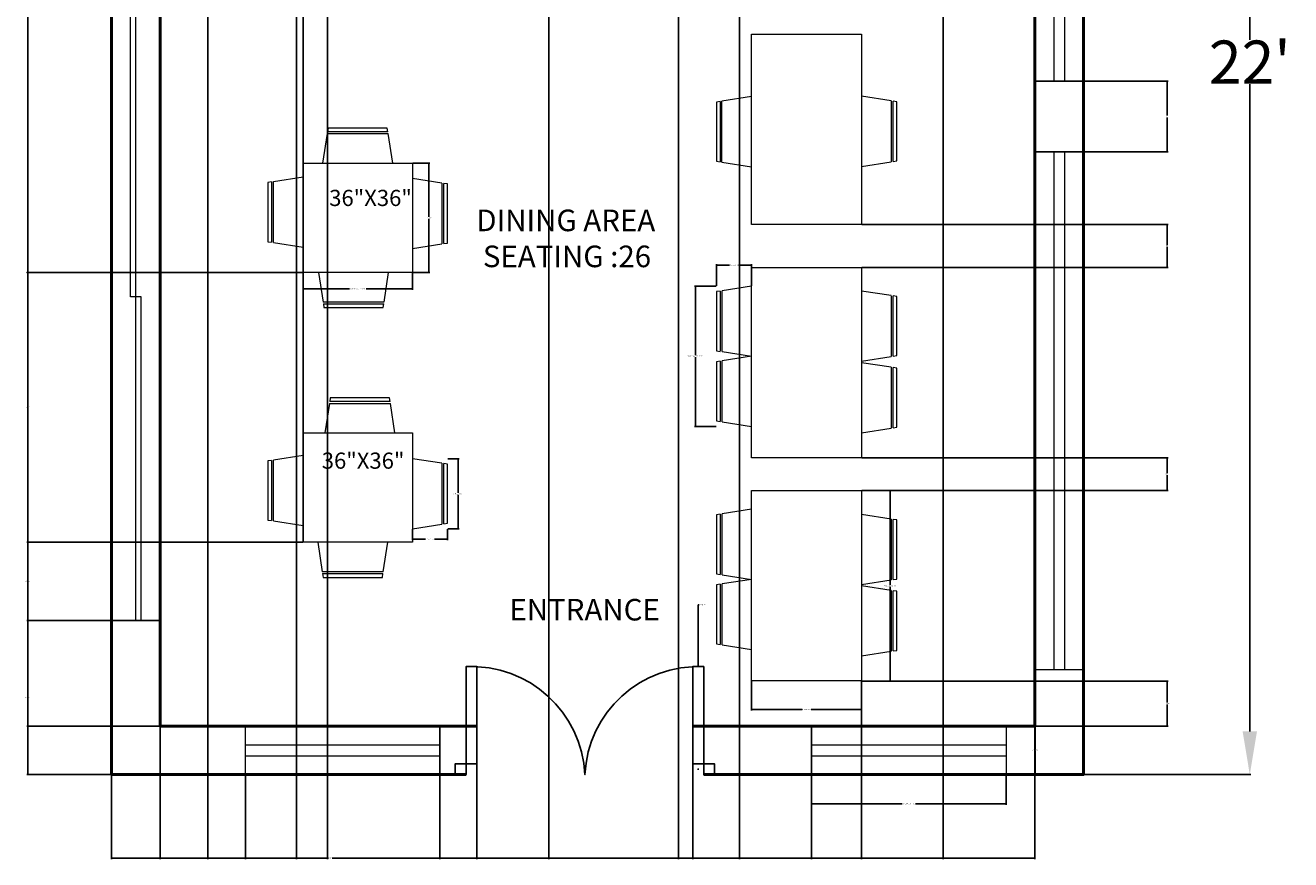
# Model space of a CAD drawing. Units: inches. Extents: x 226 to 1155, y 22 to 494.
# Tile 1 of 7: x 226 to 460, y 22 to 176. Entities that reach past the tile are written whole.
import ezdxf

# ---------------------------------------------------------------- set-up
doc = ezdxf.new("R2010")
doc.units = ezdxf.units.IN
doc.header["$MEASUREMENT"] = 0
for name, color, linetype, lineweight in [('A-ANNO-DIMS', 2, 'Continuous', 18), ('A-ANNO-TEXT', 7, 'Continuous', 18), ('A-AREA-IDEN', 7, 'Continuous', 25), ('A-DOOR', 3, 'Continuous', 25), ('A-FURN', 8, 'Continuous', 18), ('A-GLAZ', 4, 'Continuous', 18), ('A-WALL', 7, 'Continuous', 50)]:
    doc.layers.add(name, color=color, linetype=linetype, lineweight=lineweight)
doc.styles.get("Standard").update_dxf_attribs({"font": 'arial.ttf'})
doc.dimstyles.get("Standard").update_dxf_attribs({"dimtxt": 0.18, "dimasz": 0.18, "dimexe": 0.18, "dimexo": 0.0625, "dimgap": 0.09, "dimtad": 0, "dimtih": 1, "dimtoh": 1, "dimdec": 4, "dimzin": 0, "dimdsep": 46, "dimlunit": 4, "dimtxsty": 'Standard', "dimcen": 0.09, "dimadec": 0, "dimazin": 0, "dimtfac": 1, "dimtdec": 4, "dimtofl": 0, "dimtmove": 0, "dimatfit": 3, "dimfxl": 1, "dimtolj": 1, "dimtzin": 0, "dimarcsym": 0})

# ---------------------------------------------------------------- blocks, each defined once
blk = doc.blocks.new('*D8')
at = {"layer": 'A-ANNO-DIMS', "color": 0, "lineweight": -2, "transparency": 16777216}
for p, q in [((421.77, 301.63), (452.71, 301.63)), ((452.53, 293.63), (452.53, 173.74)), ((452.53, 45.63), (452.53, 165.52)), ((421.77, 37.63), (452.71, 37.63))]:
    blk.add_line(p, q, dxfattribs=at)
at = {"layer": 'A-ANNO-DIMS', "color": 0, "transparency": 16777216}
for points in [[(451.2, 293.63), (453.86, 293.63), (452.53, 301.63)], [(451.2, 45.63), (453.86, 45.63), (452.53, 37.63)]]:
    blk.add_solid(points, dxfattribs=at)
at = {"layer": 'Defpoints', "color": 0, "transparency": 16777216}
for p in [(421.71, 301.63), (421.71, 37.63), (452.53, 37.63)]:
    blk.add_point(p, dxfattribs=at)
at = {"layer": 'A-ANNO-DIMS', "color": 0, "transparency": 16777216, "insert": (452.53, 169.63), "char_height": 8, "attachment_point": 5}
blk.add_mtext("\\A1;22'", dxfattribs=at)
blk = doc.blocks.new('CHAIR-DINING')
for p, q in [((5.48, 12.14), (0, 12.99)), ((5.48, 12.13), (5.48, 0.85)), ((5.82, 0.91), (5.82, 12.08)), ((0, 0), (5.48, 0.86))]:
    blk.add_line(p, q)
blk.add_lwpolyline([(5.82, 0.91), (6.51, 1.02), (6.51, 11.98), (5.82, 12.08)])
blk = doc.blocks.new('CHAIR-DINING-PAIRED')
for p, q in [((6.51, 25.99), (1.03, 25.13)), ((0.68, 25.08), (0.68, 13.91)), ((1.03, 13.85), (1.03, 25.13)), ((0.68, 12.08), (0.68, 0.91)), ((1.03, 0.86), (1.03, 12.14)), ((1.03, 0.86), (6.51, 0))]:
    blk.add_line(p, q)
for points in [[(0.68, 25.08), (0, 24.97), (0, 14.01), (0.68, 13.9)], [(0.68, 12.08), (0, 11.98), (0, 1.02), (0.68, 0.91)], [(1.03, 13.85), (6.51, 12.99), (1.03, 12.14)]]:
    blk.add_lwpolyline(points)
blk = doc.blocks.new('TABLE-DINING-SQ')
blk.add_lwpolyline([(0, 20.25), (20.25, 20.25), (20.25, 0), (0, 0)], close=True)
blk = doc.blocks.new('TABLE-DINING-RECT')
blk.add_lwpolyline([(0, 35.29), (20.38, 35.29), (20.38, 0), (0, 0)], close=True)
blk = doc.blocks.new('WIN-36')
for p, q in [((0, 5.5), (36, 5.5)), ((0, 3.5), (36, 3.5))]:
    blk.add_line(p, q)
blk.add_lwpolyline([(36, 9), (36, 0), (0, 0), (0, 9)], close=True)
blk = doc.blocks.new('WIN-96')
for p, q in [((3.5, 96), (3.5, 0)), ((5.5, 96), (5.5, 0))]:
    blk.add_line(p, q)
blk.add_lwpolyline([(9, 96), (9, 0), (0, 0), (0, 96)], close=True)
blk = doc.blocks.new('WIN-120-SLIDING')
blk.add_lwpolyline([(9, 0), (0, 0), (0, 120), (9, 120)], close=True)
for points in [[(5.5, 0), (5.5, 60), (4.5, 60), (3.5, 60), (3.5, 120)], [(4.5, 0), (4.5, 60), (4.5, 120)]]:
    blk.add_lwpolyline(points)
blk = doc.blocks.new('*D22')
at = {"layer": 'A-ANNO-DIMS', "color": 0, "lineweight": -2, "transparency": 16777216}
for p, q in [((304, 96.16), (306.07, 96.16)), ((305.89, 95.98), (305.89, 89.85)), ((305.89, 83.35), (305.89, 89.48)), ((304, 83.17), (306.07, 83.17))]:
    blk.add_line(p, q, dxfattribs=at)
at = {"layer": 'A-ANNO-DIMS', "color": 0, "transparency": 16777216}
for points in [[(305.86, 95.98), (305.92, 95.98), (305.89, 96.16)], [(305.86, 83.35), (305.92, 83.35), (305.89, 83.17)]]:
    blk.add_solid(points, dxfattribs=at)
at = {"layer": 'Defpoints', "color": 0, "transparency": 16777216}
for p in [(303.94, 96.16), (305.89, 96.16), (303.94, 83.17)]:
    blk.add_point(p, dxfattribs=at)
at = {"layer": 'A-ANNO-DIMS', "color": 0, "transparency": 16777216, "insert": (305.89, 89.67), "char_height": 0.18, "attachment_point": 5}
blk.add_mtext('\\A1;CHAIR 1\'-1" TYP.', dxfattribs=at)
blk = doc.blocks.new('*D23')
at = {"layer": 'A-ANNO-DIMS', "color": 0, "lineweight": -2, "transparency": 16777216}
for p, q in [((297.43, 83.11), (297.43, 81.04)), ((303.94, 83.11), (303.94, 81.04)), ((297.61, 81.22), (299.84, 81.22)), ((303.76, 81.22), (301.53, 81.22))]:
    blk.add_line(p, q, dxfattribs=at)
at = {"layer": 'A-ANNO-DIMS', "color": 0, "transparency": 16777216}
for points in [[(297.61, 81.25), (297.61, 81.19), (297.43, 81.22)], [(303.76, 81.25), (303.76, 81.19), (303.94, 81.22)]]:
    blk.add_solid(points, dxfattribs=at)
at = {"layer": 'Defpoints', "color": 0, "transparency": 16777216}
for p in [(297.43, 83.17), (303.94, 83.17), (303.94, 81.22)]:
    blk.add_point(p, dxfattribs=at)
at = {"layer": 'A-ANNO-DIMS', "color": 0, "transparency": 16777216, "insert": (300.68, 81.22), "char_height": 0.18, "attachment_point": 5}
blk.add_mtext('\\A1;0\'-6 1/2" TYP.', dxfattribs=at)
blk = doc.blocks.new('*D28')
at = {"layer": 'A-ANNO-DIMS', "color": 0, "lineweight": -2, "transparency": 16777216}
for p, q in [((380.69, 90.26), (386.1, 90.26)), ((385.92, 90.08), (385.92, 72.8)), ((385.92, 55.15), (385.92, 72.44)), ((380.69, 54.97), (386.1, 54.97))]:
    blk.add_line(p, q, dxfattribs=at)
at = {"layer": 'A-ANNO-DIMS', "color": 0, "transparency": 16777216}
for points in [[(385.89, 90.08), (385.95, 90.08), (385.92, 90.26)], [(385.89, 55.15), (385.95, 55.15), (385.92, 54.97)]]:
    blk.add_solid(points, dxfattribs=at)
at = {"layer": 'Defpoints', "color": 0, "transparency": 16777216}
for p in [(380.63, 90.26), (385.92, 90.26), (380.63, 54.97)]:
    blk.add_point(p, dxfattribs=at)
at = {"layer": 'A-ANNO-DIMS', "color": 0, "transparency": 16777216, "insert": (385.92, 72.62), "char_height": 0.18, "attachment_point": 5}
blk.add_mtext('\\A1;TABLE 2\'-11 1/2" TYP.', dxfattribs=at)
blk = doc.blocks.new('*D29')
at = {"layer": 'A-ANNO-DIMS', "color": 0, "lineweight": -2, "transparency": 16777216}
for p, q in [((360.25, 54.91), (360.25, 49.5)), ((380.63, 54.91), (380.63, 49.5)), ((360.43, 49.68), (369.6, 49.68)), ((380.45, 49.68), (371.28, 49.68))]:
    blk.add_line(p, q, dxfattribs=at)
at = {"layer": 'A-ANNO-DIMS', "color": 0, "transparency": 16777216}
for points in [[(360.43, 49.71), (360.43, 49.65), (360.25, 49.68)], [(380.45, 49.71), (380.45, 49.65), (380.63, 49.68)]]:
    blk.add_solid(points, dxfattribs=at)
at = {"layer": 'Defpoints', "color": 0, "transparency": 16777216}
for p in [(360.25, 54.97), (380.63, 54.97), (380.63, 49.68)]:
    blk.add_point(p, dxfattribs=at)
at = {"layer": 'A-ANNO-DIMS', "color": 0, "transparency": 16777216, "insert": (370.44, 49.68), "char_height": 0.18, "attachment_point": 5}
blk.add_mtext('\\A1;1\'-8 1/2" TYP.', dxfattribs=at)
blk = doc.blocks.new('*D32')
at = {"layer": 'A-ANNO-DIMS', "color": 0, "lineweight": -2, "transparency": 16777216}
for p, q in [((371.38, 37.57), (371.38, 32.05)), ((407.38, 37.57), (407.38, 32.05)), ((371.56, 32.23), (388.16, 32.23)), ((407.2, 32.23), (390.61, 32.23))]:
    blk.add_line(p, q, dxfattribs=at)
at = {"layer": 'A-ANNO-DIMS', "color": 0, "transparency": 16777216}
for points in [[(371.56, 32.26), (371.56, 32.2), (371.38, 32.23)], [(407.2, 32.26), (407.2, 32.2), (407.38, 32.23)]]:
    blk.add_solid(points, dxfattribs=at)
at = {"layer": 'Defpoints', "color": 0, "transparency": 16777216}
for p in [(371.38, 37.63), (407.38, 37.63), (407.38, 32.23)]:
    blk.add_point(p, dxfattribs=at)
at = {"layer": 'A-ANNO-DIMS', "color": 0, "transparency": 16777216, "insert": (389.38, 32.23), "char_height": 0.18, "attachment_point": 5}
blk.add_mtext('\\A1;WINDOW 3\'-0" TYP.', dxfattribs=at)
blk = doc.blocks.new('*D33')
at = {"layer": 'A-ANNO-DIMS', "color": 0, "lineweight": -2, "transparency": 16777216}
for p, q in [((407.45, 46.63), (412.96, 46.63)), ((412.78, 46.45), (412.78, 42.31)), ((412.78, 37.81), (412.78, 41.95)), ((407.45, 37.63), (412.96, 37.63))]:
    blk.add_line(p, q, dxfattribs=at)
at = {"layer": 'A-ANNO-DIMS', "color": 0, "transparency": 16777216}
for points in [[(412.75, 46.45), (412.81, 46.45), (412.78, 46.63)], [(412.75, 37.81), (412.81, 37.81), (412.78, 37.63)]]:
    blk.add_solid(points, dxfattribs=at)
at = {"layer": 'Defpoints', "color": 0, "transparency": 16777216}
for p in [(407.38, 46.63), (412.78, 46.63), (407.38, 37.63)]:
    blk.add_point(p, dxfattribs=at)
at = {"layer": 'A-ANNO-DIMS', "color": 0, "transparency": 16777216, "insert": (412.78, 42.13), "char_height": 0.18, "attachment_point": 5}
blk.add_mtext('\\A1;0\'-9" TYP.', dxfattribs=at)
blk = doc.blocks.new('*D34')
at = {"layer": 'A-ANNO-DIMS', "color": 0, "lineweight": -2, "transparency": 16777216}
for p, q in [((353.68, 128.13), (349.67, 128.13)), ((349.85, 127.95), (349.85, 115.32)), ((349.85, 102.32), (349.85, 114.95)), ((353.68, 102.14), (349.67, 102.14))]:
    blk.add_line(p, q, dxfattribs=at)
at = {"layer": 'A-ANNO-DIMS', "color": 0, "transparency": 16777216}
for points in [[(349.82, 127.95), (349.88, 127.95), (349.85, 128.13)], [(349.82, 102.32), (349.88, 102.32), (349.85, 102.14)]]:
    blk.add_solid(points, dxfattribs=at)
at = {"layer": 'Defpoints', "color": 0, "transparency": 16777216}
for p in [(349.85, 128.13), (353.74, 128.13), (353.74, 102.14)]:
    blk.add_point(p, dxfattribs=at)
at = {"layer": 'A-ANNO-DIMS', "color": 0, "transparency": 16777216, "insert": (349.85, 115.14), "char_height": 0.18, "attachment_point": 5}
blk.add_mtext('\\A1;PAIRED CHAIRS 2\'-2" TYP.', dxfattribs=at)
blk = doc.blocks.new('*D35')
at = {"layer": 'A-ANNO-DIMS', "color": 0, "lineweight": -2, "transparency": 16777216}
for p, q in [((353.74, 128.19), (353.74, 132.21)), ((353.92, 132.03), (356.15, 132.03)), ((360.07, 132.03), (357.85, 132.03)), ((360.25, 128.19), (360.25, 132.21))]:
    blk.add_line(p, q, dxfattribs=at)
at = {"layer": 'A-ANNO-DIMS', "color": 0, "transparency": 16777216}
for points in [[(353.92, 132.06), (353.92, 132), (353.74, 132.03)], [(360.07, 132.06), (360.07, 132), (360.25, 132.03)]]:
    blk.add_solid(points, dxfattribs=at)
at = {"layer": 'Defpoints', "color": 0, "transparency": 16777216}
for p in [(360.25, 132.03), (353.74, 128.13), (360.25, 128.13)]:
    blk.add_point(p, dxfattribs=at)
at = {"layer": 'A-ANNO-DIMS', "color": 0, "transparency": 16777216, "insert": (357, 132.03), "char_height": 0.18, "attachment_point": 5}
blk.add_mtext('\\A1;0\'-6 1/2" TYP.', dxfattribs=at)
blk = doc.blocks.new('*D40')
at = {"layer": 'A-ANNO-DIMS', "color": 0, "lineweight": -2, "transparency": 16777216}
for p, q in [((277.18, 130.6), (277.18, 127.45)), ((297.43, 130.6), (297.43, 127.45)), ((277.36, 127.63), (285.77, 127.63)), ((297.25, 127.63), (288.84, 127.63))]:
    blk.add_line(p, q, dxfattribs=at)
at = {"layer": 'A-ANNO-DIMS', "color": 0, "transparency": 16777216}
for points in [[(277.36, 127.66), (277.36, 127.6), (277.18, 127.63)], [(297.25, 127.66), (297.25, 127.6), (297.43, 127.63)]]:
    blk.add_solid(points, dxfattribs=at)
at = {"layer": 'Defpoints', "color": 0, "transparency": 16777216}
for p in [(277.18, 130.67), (297.43, 130.67), (297.43, 127.63)]:
    blk.add_point(p, dxfattribs=at)
at = {"layer": 'A-ANNO-DIMS', "color": 0, "transparency": 16777216, "insert": (287.31, 127.63), "char_height": 0.18, "attachment_point": 5}
blk.add_mtext('\\A1;TABLE BLOCK 1\'-8" TYP.', dxfattribs=at)
blk = doc.blocks.new('*D41')
at = {"layer": 'A-ANNO-DIMS', "color": 0, "lineweight": -2, "transparency": 16777216}
for p, q in [((297.49, 150.91), (300.65, 150.91)), ((300.47, 150.73), (300.47, 140.97)), ((300.47, 130.85), (300.47, 140.61)), ((297.49, 130.67), (300.65, 130.67))]:
    blk.add_line(p, q, dxfattribs=at)
at = {"layer": 'A-ANNO-DIMS', "color": 0, "transparency": 16777216}
for points in [[(300.44, 150.73), (300.5, 150.73), (300.47, 150.91)], [(300.44, 130.85), (300.5, 130.85), (300.47, 130.67)]]:
    blk.add_solid(points, dxfattribs=at)
at = {"layer": 'Defpoints', "color": 0, "transparency": 16777216}
for p in [(297.43, 150.91), (300.47, 150.91), (297.43, 130.67)]:
    blk.add_point(p, dxfattribs=at)
at = {"layer": 'A-ANNO-DIMS', "color": 0, "transparency": 16777216, "insert": (300.47, 140.79), "char_height": 0.18, "attachment_point": 5}
blk.add_mtext('\\A1;1\'-8" TYP.', dxfattribs=at)
blk = doc.blocks.new('*D61')
at = {"layer": 'A-ANNO-DIMS', "color": 0, "lineweight": -2, "transparency": 16777216}
for p, q in [((309.38, 46.57), (309.38, 21.95)), ((349.38, 46.57), (349.38, 21.95)), ((309.56, 22.13), (329.05, 22.13)), ((349.2, 22.13), (329.71, 22.13))]:
    blk.add_line(p, q, dxfattribs=at)
at = {"layer": 'A-ANNO-DIMS', "color": 0, "transparency": 16777216}
for points in [[(309.56, 22.16), (309.56, 22.1), (309.38, 22.13)], [(349.2, 22.16), (349.2, 22.1), (349.38, 22.13)]]:
    blk.add_solid(points, dxfattribs=at)
at = {"layer": 'Defpoints', "color": 0, "transparency": 16777216}
for p in [(309.38, 46.63), (349.38, 46.63), (349.38, 22.13)]:
    blk.add_point(p, dxfattribs=at)
at = {"layer": 'A-ANNO-DIMS', "color": 0, "transparency": 16777216, "insert": (329.38, 22.13), "char_height": 0.18, "attachment_point": 5}
blk.add_mtext('\\A1;3\'-4"', dxfattribs=at)
blk = doc.blocks.new('*D62')
at = {"layer": 'A-ANNO-DIMS', "color": 0, "lineweight": -2, "transparency": 16777216}
for p, q in [((241.71, 37.57), (241.71, 21.95)), ((266.49, 37.57), (266.49, 21.95)), ((241.89, 22.13), (253.77, 22.13)), ((266.31, 22.13), (254.43, 22.13))]:
    blk.add_line(p, q, dxfattribs=at)
at = {"layer": 'A-ANNO-DIMS', "color": 0, "transparency": 16777216}
for points in [[(241.89, 22.16), (241.89, 22.1), (241.71, 22.13)], [(266.31, 22.16), (266.31, 22.1), (266.49, 22.13)]]:
    blk.add_solid(points, dxfattribs=at)
at = {"layer": 'Defpoints', "color": 0, "transparency": 16777216}
for p in [(241.71, 37.63), (266.49, 37.63), (266.49, 22.13)]:
    blk.add_point(p, dxfattribs=at)
at = {"layer": 'A-ANNO-DIMS', "color": 0, "transparency": 16777216, "insert": (254.1, 22.13), "char_height": 0.18, "attachment_point": 5}
blk.add_mtext('\\A1;2\'-1"', dxfattribs=at)
blk = doc.blocks.new('*D63')
at = {"layer": 'A-ANNO-DIMS', "color": 0, "lineweight": -2, "transparency": 16777216}
for p, q in [((302.49, 46.57), (302.49, 21.95)), ((309.38, 46.57), (309.38, 21.95)), ((302.67, 22.13), (305.6, 22.13)), ((309.2, 22.13), (306.26, 22.13))]:
    blk.add_line(p, q, dxfattribs=at)
at = {"layer": 'A-ANNO-DIMS', "color": 0, "transparency": 16777216}
for points in [[(302.67, 22.16), (302.67, 22.1), (302.49, 22.13)], [(309.2, 22.16), (309.2, 22.1), (309.38, 22.13)]]:
    blk.add_solid(points, dxfattribs=at)
at = {"layer": 'Defpoints', "color": 0, "transparency": 16777216}
for p in [(302.49, 46.63), (309.38, 46.63), (309.38, 22.13)]:
    blk.add_point(p, dxfattribs=at)
at = {"layer": 'A-ANNO-DIMS', "color": 0, "transparency": 16777216, "insert": (305.93, 22.13), "char_height": 0.18, "attachment_point": 5}
blk.add_mtext('\\A1;0\'-7"', dxfattribs=at)
blk = doc.blocks.new('*D64')
at = {"layer": 'A-ANNO-DIMS', "color": 0, "lineweight": -2, "transparency": 16777216}
for p, q in [((349.38, 46.57), (349.38, 21.95)), ((371.38, 46.57), (371.38, 21.95)), ((349.56, 22.13), (359.99, 22.13)), ((371.2, 22.13), (360.77, 22.13))]:
    blk.add_line(p, q, dxfattribs=at)
at = {"layer": 'A-ANNO-DIMS', "color": 0, "transparency": 16777216}
for points in [[(349.56, 22.16), (349.56, 22.1), (349.38, 22.13)], [(371.2, 22.16), (371.2, 22.1), (371.38, 22.13)]]:
    blk.add_solid(points, dxfattribs=at)
at = {"layer": 'Defpoints', "color": 0, "transparency": 16777216}
for p in [(349.38, 46.63), (371.38, 46.63), (371.38, 22.13)]:
    blk.add_point(p, dxfattribs=at)
at = {"layer": 'A-ANNO-DIMS', "color": 0, "transparency": 16777216, "insert": (360.38, 22.13), "char_height": 0.18, "attachment_point": 5}
blk.add_mtext('\\A1;1\'-10"', dxfattribs=at)
blk = doc.blocks.new('*D65')
at = {"layer": 'A-ANNO-DIMS', "color": 0, "lineweight": -2, "transparency": 16777216}
for p, q in [((241.64, 66.17), (226.03, 66.17)), ((226.21, 65.99), (226.21, 52.08)), ((226.21, 37.81), (226.21, 51.72)), ((241.64, 37.63), (226.03, 37.63))]:
    blk.add_line(p, q, dxfattribs=at)
at = {"layer": 'A-ANNO-DIMS', "color": 0, "transparency": 16777216}
for points in [[(226.18, 65.99), (226.24, 65.99), (226.21, 66.17)], [(226.18, 37.81), (226.24, 37.81), (226.21, 37.63)]]:
    blk.add_solid(points, dxfattribs=at)
at = {"layer": 'Defpoints', "color": 0, "transparency": 16777216}
for p in [(226.21, 66.17), (241.71, 66.17), (241.71, 37.63)]:
    blk.add_point(p, dxfattribs=at)
at = {"layer": 'A-ANNO-DIMS', "color": 0, "transparency": 16777216, "insert": (226.21, 51.9), "char_height": 0.18, "attachment_point": 5}
blk.add_mtext('\\A1;2\'-4 1/2"', dxfattribs=at)
blk = doc.blocks.new('*D67')
at = {"layer": 'A-ANNO-DIMS', "color": 0, "lineweight": -2, "transparency": 16777216}
for p, q in [((250.64, 214.63), (226.03, 214.63)), ((226.21, 214.45), (226.21, 130.81)), ((226.21, 46.81), (226.21, 130.45)), ((250.64, 46.63), (226.03, 46.63))]:
    blk.add_line(p, q, dxfattribs=at)
at = {"layer": 'A-ANNO-DIMS', "color": 0, "transparency": 16777216}
for points in [[(226.18, 214.45), (226.24, 214.45), (226.21, 214.63)], [(226.18, 46.81), (226.24, 46.81), (226.21, 46.63)]]:
    blk.add_solid(points, dxfattribs=at)
at = {"layer": 'Defpoints', "color": 0, "transparency": 16777216}
for p in [(226.21, 214.63), (250.71, 214.63), (250.71, 46.63)]:
    blk.add_point(p, dxfattribs=at)
at = {"layer": 'A-ANNO-DIMS', "color": 0, "transparency": 16777216, "insert": (226.21, 130.63), "char_height": 0.18, "attachment_point": 5}
blk.add_mtext('\\A1;14\'-0"', dxfattribs=at)
blk = doc.blocks.new('*D68')
at = {"layer": 'A-ANNO-DIMS', "color": 0, "lineweight": -2, "transparency": 16777216}
for p, q in [((277.12, 130.67), (226.03, 130.67)), ((226.21, 130.49), (226.21, 105.86)), ((226.21, 80.87), (226.21, 105.5)), ((277.12, 80.69), (226.03, 80.69))]:
    blk.add_line(p, q, dxfattribs=at)
at = {"layer": 'A-ANNO-DIMS', "color": 0, "transparency": 16777216}
for points in [[(226.18, 130.49), (226.24, 130.49), (226.21, 130.67)], [(226.18, 80.87), (226.24, 80.87), (226.21, 80.69)]]:
    blk.add_solid(points, dxfattribs=at)
at = {"layer": 'Defpoints', "color": 0, "transparency": 16777216}
for p in [(226.21, 130.67), (277.18, 130.67), (277.18, 80.69)]:
    blk.add_point(p, dxfattribs=at)
at = {"layer": 'A-ANNO-DIMS', "color": 0, "transparency": 16777216, "insert": (226.21, 105.68), "char_height": 0.18, "attachment_point": 5}
blk.add_mtext('\\A1;4\'-2"', dxfattribs=at)
blk = doc.blocks.new('*D69')
at = {"layer": 'A-ANNO-DIMS', "color": 0, "lineweight": -2, "transparency": 16777216}
for p, q in [((250.71, 46.69), (250.71, 317.31)), ((250.89, 317.13), (263.4, 317.13)), ((277, 317.13), (264.48, 317.13)), ((277.18, 80.75), (277.18, 317.31))]:
    blk.add_line(p, q, dxfattribs=at)
at = {"layer": 'A-ANNO-DIMS', "color": 0, "transparency": 16777216}
for points in [[(250.89, 317.16), (250.89, 317.1), (250.71, 317.13)], [(277, 317.16), (277, 317.1), (277.18, 317.13)]]:
    blk.add_solid(points, dxfattribs=at)
at = {"layer": 'Defpoints', "color": 0, "transparency": 16777216}
for p in [(277.18, 317.13), (277.18, 80.69), (250.71, 46.63)]:
    blk.add_point(p, dxfattribs=at)
at = {"layer": 'A-ANNO-DIMS', "color": 0, "transparency": 16777216, "insert": (263.94, 317.13), "char_height": 0.18, "attachment_point": 5}
blk.add_mtext('\\A1;2\'-2 1/2"', dxfattribs=at)
blk = doc.blocks.new('*D70')
at = {"layer": 'A-ANNO-DIMS', "color": 0, "lineweight": -2, "transparency": 16777216}
for p, q in [((380.63, 54.91), (380.63, 21.95)), ((412.71, 46.57), (412.71, 21.95)), ((380.81, 22.13), (396.34, 22.13)), ((412.53, 22.13), (397, 22.13))]:
    blk.add_line(p, q, dxfattribs=at)
at = {"layer": 'A-ANNO-DIMS', "color": 0, "transparency": 16777216}
for points in [[(380.81, 22.16), (380.81, 22.1), (380.63, 22.13)], [(412.53, 22.16), (412.53, 22.1), (412.71, 22.13)]]:
    blk.add_solid(points, dxfattribs=at)
at = {"layer": 'Defpoints', "color": 0, "transparency": 16777216}
for p in [(380.63, 54.97), (412.71, 46.63), (412.71, 22.13)]:
    blk.add_point(p, dxfattribs=at)
at = {"layer": 'A-ANNO-DIMS', "color": 0, "transparency": 16777216, "insert": (396.67, 22.13), "char_height": 0.18, "attachment_point": 5}
blk.add_mtext('\\A1;2\'-8"', dxfattribs=at)
blk = doc.blocks.new('*D71')
at = {"layer": 'A-ANNO-DIMS', "color": 0, "lineweight": -2, "transparency": 16777216}
for p, q in [((241.71, 301.57), (241.71, 21.95)), ((322.71, 301.57), (322.71, 21.95)), ((241.89, 22.13), (281.88, 22.13)), ((322.53, 22.13), (282.54, 22.13))]:
    blk.add_line(p, q, dxfattribs=at)
at = {"layer": 'A-ANNO-DIMS', "color": 0, "transparency": 16777216}
for points in [[(241.89, 22.16), (241.89, 22.1), (241.71, 22.13)], [(322.53, 22.16), (322.53, 22.1), (322.71, 22.13)]]:
    blk.add_solid(points, dxfattribs=at)
at = {"layer": 'Defpoints', "color": 0, "transparency": 16777216}
for p in [(241.71, 301.63), (322.71, 301.63), (322.71, 22.13)]:
    blk.add_point(p, dxfattribs=at)
at = {"layer": 'A-ANNO-DIMS', "color": 0, "transparency": 16777216, "insert": (282.21, 22.13), "char_height": 0.18, "attachment_point": 5}
blk.add_mtext('\\A1;6\'-9"', dxfattribs=at)
blk = doc.blocks.new('*D72')
at = {"layer": 'A-ANNO-DIMS', "color": 0, "lineweight": -2, "transparency": 16777216}
for p, q in [((322.71, 301.57), (322.71, 21.95)), ((346.71, 301.57), (346.71, 21.95)), ((322.89, 22.13), (334.38, 22.13)), ((346.53, 22.13), (335.04, 22.13))]:
    blk.add_line(p, q, dxfattribs=at)
at = {"layer": 'A-ANNO-DIMS', "color": 0, "transparency": 16777216}
for points in [[(322.89, 22.16), (322.89, 22.1), (322.71, 22.13)], [(346.53, 22.16), (346.53, 22.1), (346.71, 22.13)]]:
    blk.add_solid(points, dxfattribs=at)
at = {"layer": 'Defpoints', "color": 0, "transparency": 16777216}
for p in [(322.71, 301.63), (346.71, 301.63), (346.71, 22.13)]:
    blk.add_point(p, dxfattribs=at)
at = {"layer": 'A-ANNO-DIMS', "color": 0, "transparency": 16777216, "insert": (334.71, 22.13), "char_height": 0.18, "attachment_point": 5}
blk.add_mtext('\\A1;2\'-0"', dxfattribs=at)
blk = doc.blocks.new('*D73')
at = {"layer": 'A-ANNO-DIMS', "color": 0, "lineweight": -2, "transparency": 16777216}
for p, q in [((380.69, 54.97), (437.39, 54.97)), ((437.21, 54.79), (437.21, 50.98)), ((437.21, 46.81), (437.21, 50.62)), ((412.77, 46.63), (437.39, 46.63))]:
    blk.add_line(p, q, dxfattribs=at)
at = {"layer": 'A-ANNO-DIMS', "color": 0, "transparency": 16777216}
for points in [[(437.18, 54.79), (437.24, 54.79), (437.21, 54.97)], [(437.18, 46.81), (437.24, 46.81), (437.21, 46.63)]]:
    blk.add_solid(points, dxfattribs=at)
at = {"layer": 'Defpoints', "color": 0, "transparency": 16777216}
for p in [(380.63, 54.97), (437.21, 54.97), (412.71, 46.63)]:
    blk.add_point(p, dxfattribs=at)
at = {"layer": 'A-ANNO-DIMS', "color": 0, "transparency": 16777216, "insert": (437.21, 50.8), "char_height": 0.18, "attachment_point": 5}
blk.add_mtext('\\A1;0\'-8 1/2"', dxfattribs=at)
blk = doc.blocks.new('*D74')
at = {"layer": 'A-ANNO-DIMS', "color": 0, "lineweight": -2, "transparency": 16777216}
for p, q in [((380.69, 96.31), (437.39, 96.31)), ((437.21, 96.13), (437.21, 93.47)), ((437.21, 90.44), (437.21, 93.1)), ((380.69, 90.26), (437.39, 90.26))]:
    blk.add_line(p, q, dxfattribs=at)
at = {"layer": 'A-ANNO-DIMS', "color": 0, "transparency": 16777216}
for points in [[(437.18, 96.13), (437.24, 96.13), (437.21, 96.31)], [(437.18, 90.44), (437.24, 90.44), (437.21, 90.26)]]:
    blk.add_solid(points, dxfattribs=at)
at = {"layer": 'Defpoints', "color": 0, "transparency": 16777216}
for p in [(380.63, 96.31), (437.21, 96.31), (380.63, 90.26)]:
    blk.add_point(p, dxfattribs=at)
at = {"layer": 'A-ANNO-DIMS', "color": 0, "transparency": 16777216, "insert": (437.21, 93.28), "char_height": 0.18, "attachment_point": 5}
blk.add_mtext('\\A1;0\'-6"', dxfattribs=at)
blk = doc.blocks.new('*D75')
at = {"layer": 'A-ANNO-DIMS', "color": 0, "lineweight": -2, "transparency": 16777216}
for p, q in [((380.69, 139.55), (437.39, 139.55)), ((437.21, 139.37), (437.21, 135.75)), ((437.21, 131.78), (437.21, 135.39)), ((380.69, 131.6), (437.39, 131.6))]:
    blk.add_line(p, q, dxfattribs=at)
at = {"layer": 'A-ANNO-DIMS', "color": 0, "transparency": 16777216}
for points in [[(437.18, 139.37), (437.24, 139.37), (437.21, 139.55)], [(437.18, 131.78), (437.24, 131.78), (437.21, 131.6)]]:
    blk.add_solid(points, dxfattribs=at)
at = {"layer": 'Defpoints', "color": 0, "transparency": 16777216}
for p in [(380.63, 139.55), (437.21, 139.55), (380.63, 131.6)]:
    blk.add_point(p, dxfattribs=at)
at = {"layer": 'A-ANNO-DIMS', "color": 0, "transparency": 16777216, "insert": (437.21, 135.57), "char_height": 0.18, "attachment_point": 5}
blk.add_mtext('\\A1;0\'-8"', dxfattribs=at)
blk = doc.blocks.new('*D76')
at = {"layer": 'A-ANNO-DIMS', "color": 0, "lineweight": -2, "transparency": 16777216}
for p, q in [((412.77, 166.11), (437.39, 166.11)), ((437.21, 165.93), (437.21, 159.74)), ((437.21, 153.19), (437.21, 159.38)), ((412.77, 153.01), (437.39, 153.01))]:
    blk.add_line(p, q, dxfattribs=at)
at = {"layer": 'A-ANNO-DIMS', "color": 0, "transparency": 16777216}
for points in [[(437.18, 165.93), (437.24, 165.93), (437.21, 166.11)], [(437.18, 153.19), (437.24, 153.19), (437.21, 153.01)]]:
    blk.add_solid(points, dxfattribs=at)
at = {"layer": 'Defpoints', "color": 0, "transparency": 16777216}
for p in [(412.71, 166.11), (437.21, 166.11), (412.71, 153.01)]:
    blk.add_point(p, dxfattribs=at)
at = {"layer": 'A-ANNO-DIMS', "color": 0, "transparency": 16777216, "insert": (437.21, 159.56), "char_height": 0.18, "attachment_point": 5}
blk.add_mtext('\\A1;1\'-1"', dxfattribs=at)
blk = doc.blocks.new('*D77')
at = {"layer": 'A-ANNO-DIMS', "color": 0, "lineweight": -2, "transparency": 16777216}
for p, q in [((277.12, 80.69), (226.03, 80.69)), ((226.21, 80.51), (226.21, 73.61)), ((226.21, 66.35), (226.21, 73.24)), ((250.64, 66.17), (226.03, 66.17))]:
    blk.add_line(p, q, dxfattribs=at)
at = {"layer": 'A-ANNO-DIMS', "color": 0, "transparency": 16777216}
for points in [[(226.18, 80.51), (226.24, 80.51), (226.21, 80.69)], [(226.18, 66.35), (226.24, 66.35), (226.21, 66.17)]]:
    blk.add_solid(points, dxfattribs=at)
at = {"layer": 'Defpoints', "color": 0, "transparency": 16777216}
for p in [(226.21, 80.69), (277.18, 80.69), (250.71, 66.17)]:
    blk.add_point(p, dxfattribs=at)
at = {"layer": 'A-ANNO-DIMS', "color": 0, "transparency": 16777216, "insert": (226.21, 73.43), "char_height": 0.18, "attachment_point": 5}
blk.add_mtext('\\A1;1\'-2 1/2"', dxfattribs=at)
blk = doc.blocks.new('*D79')
at = {"layer": 'A-ANNO-DIMS', "color": 0, "lineweight": -2, "transparency": 16777216}
for p, q in [((250.71, 186.1), (250.71, 21.95)), ((259.54, 180.86), (259.54, 21.95)), ((250.89, 22.13), (254.79, 22.13)), ((259.36, 22.13), (255.45, 22.13))]:
    blk.add_line(p, q, dxfattribs=at)
at = {"layer": 'A-ANNO-DIMS', "color": 0, "transparency": 16777216}
for points in [[(250.89, 22.16), (250.89, 22.1), (250.71, 22.13)], [(259.36, 22.16), (259.36, 22.1), (259.54, 22.13)]]:
    blk.add_solid(points, dxfattribs=at)
at = {"layer": 'Defpoints', "color": 0, "transparency": 16777216}
for p in [(250.71, 186.17), (259.54, 180.93), (259.54, 22.13)]:
    blk.add_point(p, dxfattribs=at)
at = {"layer": 'A-ANNO-DIMS', "color": 0, "transparency": 16777216, "insert": (255.12, 22.13), "char_height": 0.18, "attachment_point": 5}
blk.add_mtext('\\A1;0\'-9"', dxfattribs=at)
blk = doc.blocks.new('*D80')
at = {"layer": 'A-ANNO-DIMS', "color": 0, "lineweight": -2, "transparency": 16777216}
for p, q in [((275.98, 180.86), (275.98, 21.95)), ((281.68, 180.86), (281.68, 21.95)), ((276.16, 22.13), (278.29, 22.13)), ((281.5, 22.13), (279.37, 22.13))]:
    blk.add_line(p, q, dxfattribs=at)
at = {"layer": 'A-ANNO-DIMS', "color": 0, "transparency": 16777216}
for points in [[(276.16, 22.16), (276.16, 22.1), (275.98, 22.13)], [(281.5, 22.16), (281.5, 22.1), (281.68, 22.13)]]:
    blk.add_solid(points, dxfattribs=at)
at = {"layer": 'Defpoints', "color": 0, "transparency": 16777216}
for p in [(275.98, 180.93), (281.68, 180.93), (281.68, 22.13)]:
    blk.add_point(p, dxfattribs=at)
at = {"layer": 'A-ANNO-DIMS', "color": 0, "transparency": 16777216, "insert": (278.83, 22.13), "char_height": 0.18, "attachment_point": 5}
blk.add_mtext('\\A1;0\'-5 1/2"', dxfattribs=at)
blk = doc.blocks.new('*D81')
at = {"layer": 'A-ANNO-DIMS', "color": 0, "lineweight": -2, "transparency": 16777216}
for p, q in [((358.02, 198.75), (358.02, 21.95)), ((412.71, 198.75), (412.71, 21.95)), ((358.2, 22.13), (384.82, 22.13)), ((412.53, 22.13), (385.91, 22.13))]:
    blk.add_line(p, q, dxfattribs=at)
at = {"layer": 'A-ANNO-DIMS', "color": 0, "transparency": 16777216}
for points in [[(358.2, 22.16), (358.2, 22.1), (358.02, 22.13)], [(412.53, 22.16), (412.53, 22.1), (412.71, 22.13)]]:
    blk.add_solid(points, dxfattribs=at)
at = {"layer": 'Defpoints', "color": 0, "transparency": 16777216}
for p in [(358.02, 198.82), (412.71, 198.82), (412.71, 22.13)]:
    blk.add_point(p, dxfattribs=at)
at = {"layer": 'A-ANNO-DIMS', "color": 0, "transparency": 16777216, "insert": (385.36, 22.13), "char_height": 0.18, "attachment_point": 5}
blk.add_mtext('\\A1;4\'-6 1/2"', dxfattribs=at)
blk = doc.blocks.new('*D84')
at = {"layer": 'A-ANNO-DIMS', "color": 0, "lineweight": -2, "transparency": 16777216}
for p, q in [((412.71, 292.57), (412.71, 21.95)), ((395.71, 275.57), (395.71, 21.95)), ((395.89, 22.13), (403.89, 22.13)), ((412.53, 22.13), (404.53, 22.13))]:
    blk.add_line(p, q, dxfattribs=at)
at = {"layer": 'A-ANNO-DIMS', "color": 0, "transparency": 16777216}
for points in [[(395.89, 22.16), (395.89, 22.1), (395.71, 22.13)], [(412.53, 22.16), (412.53, 22.1), (412.71, 22.13)]]:
    blk.add_solid(points, dxfattribs=at)
at = {"layer": 'Defpoints', "color": 0, "transparency": 16777216}
for p in [(412.71, 292.63), (395.71, 275.63), (412.71, 22.13)]:
    blk.add_point(p, dxfattribs=at)
at = {"layer": 'A-ANNO-DIMS', "color": 0, "transparency": 16777216, "insert": (404.21, 22.13), "char_height": 0.18, "attachment_point": 5}
blk.add_mtext('\\A1;1\'-5"', dxfattribs=at)
blk = doc.blocks.new('*D119')
at = {"layer": 'A-ANNO-DIMS', "color": 0, "lineweight": -2, "transparency": 16777216}
for p, q in [((350.56, 69.07), (350.38, 69.07)), ((350.38, 69.07), (350.38, 57.84)), ((350.29, 38.63), (350.47, 38.63)), ((350.38, 38.54), (350.38, 38.72))]:
    blk.add_line(p, q, dxfattribs=at)
at = {"layer": 'A-ANNO-DIMS', "color": 0, "transparency": 16777216}
blk.add_solid([(350.35, 57.84), (350.41, 57.84), (350.38, 57.66)], dxfattribs=at)
at = {"layer": 'Defpoints', "color": 0, "transparency": 16777216}
for p in [(350.38, 57.66), (350.38, 38.63)]:
    blk.add_point(p, dxfattribs=at)
at = {"layer": 'A-ANNO-DIMS', "color": 0, "transparency": 16777216, "insert": (351.17, 69.07), "char_height": 0.18, "attachment_point": 5}
blk.add_mtext('\\A1;4X R1\'-7"', dxfattribs=at)

msp = doc.modelspace()

# ---------------------------------------------------------------- linework, layer by layer
at = {"layer": 'A-DOOR'}
for p, q in [((305.38052, 37.62988), (307.38052, 37.62988)), ((353.38052, 37.62988), (351.38052, 37.62988))]:
    msp.add_line(p, q, dxfattribs=at)
msp.add_lwpolyline([(349.38052, 57.62988, -0.02629759), (351.38052, 57.62988), (349.38052, 57.62988), (349.38052, 39.62988), (351.38052, 39.62988), (351.38052, 57.62988, 0.414213562), (329.38052, 37.62988, 0.414213562), (307.38052, 57.62988), (307.38052, 39.62988), (309.38052, 39.62988), (309.38052, 57.62988), (307.38052, 57.62988, -0.02629759), (309.38052, 57.62988)], format="xyb", dxfattribs=at)
for points in [[(305.38052, 37.62988), (307.38052, 37.62988), (307.38052, 39.62988), (305.38052, 39.62988)], [(329.38052, 37.62988), (329.38052, 37.62988)], [(329.38052, 37.62988), (329.38052, 37.62988)], [(353.38052, 37.62988), (351.38052, 37.62988), (351.38052, 39.62988), (353.38052, 39.62988)]]:
    msp.add_lwpolyline(points, close=True, dxfattribs=at)
at = {"layer": 'A-WALL'}
for points in [[(307.38052, 37.62988), (241.70585, 37.62988), (241.70585, 301.62988), (421.70585, 301.62988), (421.70585, 37.62988), (351.38052, 37.62988)], [(309.38052, 46.62988), (250.70585, 46.62988), (250.70585, 292.62988), (312.70585, 292.62988), (312.70585, 236.41817)], [(364.70585, 214.62988), (364.70585, 292.62988), (412.70585, 292.62988), (412.70585, 46.62988), (349.38052, 46.62988)]]:
    msp.add_lwpolyline(points, dxfattribs=at)

# ---------------------------------------------------------------- block references
at = {"layer": 'A-FURN'}
for name, p in [('TABLE-DINING-RECT', (360.252, 139.546)), ('CHAIR-DINING', (380.62783, 150.31343)), ('TABLE-DINING-SQ', (277.183, 130.666)), ('CHAIR-DINING', (297.43, 135.095)), ('TABLE-DINING-RECT', (360.252, 96.3054)), ('CHAIR-DINING-PAIRED', (353.744, 102.144)), ('CHAIR-DINING', (380.62783, 114.22795)), ('CHAIR-DINING', (380.62783, 100.95729)), ('TABLE-DINING-SQ', (277.183, 80.6867)), ('CHAIR-DINING', (297.43, 83.1705)), ('TABLE-DINING-RECT', (360.252, 54.97312)), ('CHAIR-DINING-PAIRED', (353.744, 60.81107)), ('CHAIR-DINING', (380.62783, 72.8397)), ('CHAIR-DINING', (380.62783, 59.62502))]:
    msp.add_blockref(name, p, dxfattribs=at)
for p, rotation in [((360.25217, 163.25133), 180), ((293.79231, 150.91311), 90.00000000000006), ((277.1826, 148.34092), 180), ((280.0312, 130.66571), 269.9999999999996), ((294.20244, 100.93381), 90.00000000000006), ((277.1826, 96.75753), 180), ((279.88672, 80.68641), 269.9999999999997)]:
    msp.add_blockref('CHAIR-DINING', p, dxfattribs=dict(at, rotation=rotation))
at = {"layer": 'A-GLAZ', "rotation": 270}
msp.add_blockref('WIN-36', (412.70597, 202.11457), dxfattribs=at)
at = {"layer": 'A-GLAZ'}
for name, p in [('WIN-120-SLIDING', (241.706, 66.167)), ('WIN-96', (412.706, 57.01)), ('WIN-36', (266.486, 37.63)), ('WIN-36', (371.38448, 37.63))]:
    msp.add_blockref(name, p, dxfattribs=at)

# ---------------------------------------------------------------- texts
at = {"layer": 'A-ANNO-TEXT', "char_height": 3, "attachment_point": 1}
for width, insert in [(12.1239596, (282.01805, 145.9715)), (16.7887975, (280.64093, 97.29759))]:
    msp.add_mtext_dynamic_manual_height_columns('36"X36"', width=width, gutter_width=1, heights=[0], dxfattribs=dict(at, insert=insert))
at = {"layer": 'A-AREA-IDEN', "char_height": 4, "attachment_point": 1}
for s, width, insert in [('DINING AREA\\P SEATING :26', 37.218979, (309.26491, 142.30778)), ('ENTRANCE', 33.9775973, (315.40292, 70.18136))]:
    msp.add_mtext_dynamic_manual_height_columns(s, width=width, gutter_width=1, heights=[0], dxfattribs=dict(at, insert=insert))

# ---------------------------------------------------------------- dimensions: what is measured, and where the dimension line sits
at = {"layer": 'A-ANNO-DIMS'}
for base, p1, p2, picture, middle in [((277.18287, 317.12988), (250.70585, 46.62988), (277.18287, 80.68669), '*D69', (263.94436, 317.12988)), ((322.7094, 22.12988), (241.70585, 301.62988), (322.7094, 301.62988), '*D71', (282.20762, 22.12988)), ((346.7094, 22.12988), (322.7094, 301.62988), (346.7094, 301.62988), '*D72', (334.7094, 22.12988)), ((412.70584, 22.12988), (395.70585, 275.62988), (412.70584, 292.62988), '*D84', (404.20584, 22.12988)), ((412.70584, 22.12988), (358.02219, 198.81719), (412.70584, 198.81719), '*D81', (385.36402, 22.12988)), ((259.53617, 22.12988), (250.70585, 186.1667), (259.53617, 180.92618), '*D79', (255.12101, 22.12988)), ((281.67698, 22.12988), (275.98461, 180.92618), (281.67698, 180.92618), '*D80', (278.8308, 22.12988)), ((412.70584, 22.12988), (380.62756, 54.97308), (412.70584, 46.62988), '*D70', (396.6667, 22.12988)), ((309.38052, 22.12988), (302.48629, 46.62988), (309.38052, 46.62988), '*D63', (305.9334, 22.12988)), ((349.38052, 22.12988), (309.38052, 46.62988), (349.38052, 46.62988), '*D61', (329.38052, 22.12988)), ((371.38477, 22.12988), (349.38052, 46.62988), (371.38477, 46.62988), '*D64', (360.38265, 22.12988)), ((266.48629, 22.12988), (241.70585, 37.62988), (266.48629, 37.62988), '*D62', (254.09607, 22.12988))]:
    dim = msp.add_linear_dim(base=base, p1=p1, p2=p2, dimstyle='Standard', override={"dimdec": 1, "dimlfac": 1, "dimrnd": 0, "dimzin": 1, "dimdsep": 46, "dimlunit": 4, "dimfrac": 2}, dxfattribs=at)
    dim.commit()
    dim.dimension.update_dxf_attribs({"geometry": picture, "text_midpoint": middle})
for base, p1, p2, override, picture, middle in [((452.53152, 37.62988), (421.70585, 301.62988), (421.70585, 37.62988), {"dimtxt": 8, "dimasz": 8, "dimclrd": 0, "dimclre": 0, "dimclrt": 0}, '*D8', (452.53152, 169.62988)), ((226.20585, 214.62988), (250.70585, 46.62988), (250.70585, 214.62988), {"dimdec": 1, "dimlfac": 1, "dimrnd": 0, "dimzin": 1, "dimdsep": 46, "dimlunit": 4, "dimfrac": 2}, '*D67', (226.20585, 130.62988)), ((437.20585, 166.11428), (412.70584, 153.00964), (412.70584, 166.11428), {"dimdec": 1, "dimlfac": 1, "dimrnd": 0, "dimzin": 1, "dimdsep": 46, "dimlunit": 4, "dimfrac": 2}, '*D76', (437.20585, 159.56196)), ((437.20585, 139.54596), (380.62756, 131.59608), (380.62756, 139.54596), {"dimdec": 1, "dimlfac": 1, "dimrnd": 0, "dimzin": 1, "dimdsep": 46, "dimlunit": 4, "dimfrac": 2}, '*D75', (437.20585, 135.57102)), ((226.20585, 130.66598), (277.18287, 80.68669), (277.18287, 130.66598), {"dimdec": 1, "dimlfac": 1, "dimrnd": 0, "dimzin": 1, "dimdsep": 46, "dimlunit": 4, "dimfrac": 2}, '*D68', (226.20585, 105.67634)), ((437.20585, 96.30536), (380.62756, 90.2638), (380.62756, 96.30536), {"dimdec": 1, "dimlfac": 1, "dimrnd": 0, "dimzin": 1, "dimdsep": 46, "dimlunit": 4, "dimfrac": 2}, '*D74', (437.20585, 93.28458)), ((226.20585, 80.68669), (250.70585, 66.1667), (277.18287, 80.68669), {"dimdec": 1, "dimlfac": 1, "dimrnd": 0, "dimzin": 1, "dimdsep": 46, "dimlunit": 4, "dimfrac": 2}, '*D77', (226.20585, 73.4267)), ((226.20585, 66.1667), (241.70585, 37.62988), (241.70585, 66.1667), {"dimdec": 1, "dimlfac": 1, "dimrnd": 0, "dimzin": 1, "dimdsep": 46, "dimlunit": 4, "dimfrac": 2}, '*D65', (226.20585, 51.89829)), ((437.20585, 54.97308), (412.70584, 46.62988), (380.62756, 54.97308), {"dimdec": 1, "dimlfac": 1, "dimrnd": 0, "dimzin": 1, "dimdsep": 46, "dimlunit": 4, "dimfrac": 2}, '*D73', (437.20585, 50.80148))]:
    dim = msp.add_linear_dim(base=base, p1=p1, p2=p2, angle=90, dimstyle='Standard', override=override, dxfattribs=at)
    dim.commit()
    dim.dimension.update_dxf_attribs({"geometry": picture, "text_midpoint": middle})
for base, p1, p2, text, picture, middle in [((300.46675, 150.91283), (297.42972, 130.66598), (297.42972, 150.91283), '<> TYP.', '*D41', (300.46675, 140.78941)), ((349.84586, 128.13057), (353.7438, 102.14427), (353.7438, 128.13057), 'PAIRED CHAIRS <> TYP.', '*D34', (349.84586, 115.13742)), ((305.88734, 96.16393), (303.93837, 83.17078), (303.93837, 96.16393), 'CHAIR <> TYP.', '*D22', (305.88734, 89.66735)), ((385.92116, 90.2638), (380.62756, 54.97308), (380.62756, 90.2638), 'TABLE <> TYP.', '*D28', (385.92116, 72.61844)), ((412.78477, 46.62988), (407.38477, 37.62988), (407.38477, 46.62988), '<> TYP.', '*D33', (412.78477, 42.12988))]:
    dim = msp.add_linear_dim(base=base, p1=p1, p2=p2, angle=90, text=text, dimstyle='Standard', override={"dimdec": 1, "dimlfac": 1, "dimrnd": 0, "dimzin": 1, "dimdsep": 46, "dimlunit": 4, "dimfrac": 2}, dxfattribs=at)
    dim.commit()
    dim.dimension.update_dxf_attribs({"geometry": picture, "text_midpoint": middle})
for base, p1, p2, text, picture, middle in [((360.25245, 132.02851), (353.7438, 128.13057), (360.25245, 128.13057), '<> TYP.', '*D35', (356.99813, 132.02851)), ((297.42972, 127.62896), (277.18287, 130.66598), (297.42972, 130.66598), 'TABLE BLOCK <> TYP.', '*D40', (287.3063, 127.62896)), ((303.93837, 81.22181), (297.42972, 83.17078), (303.93837, 83.17078), '<> TYP.', '*D23', (300.68405, 81.22181)), ((380.62756, 49.67948), (360.25245, 54.97308), (380.62756, 54.97308), '<> TYP.', '*D29', (370.44, 49.67948)), ((407.38477, 32.22988), (371.38477, 37.62988), (407.38477, 37.62988), 'WINDOW <> TYP.', '*D32', (389.38477, 32.22988))]:
    dim = msp.add_linear_dim(base=base, p1=p1, p2=p2, text=text, dimstyle='Standard', override={"dimdec": 1, "dimlfac": 1, "dimrnd": 0, "dimzin": 1, "dimdsep": 46, "dimlunit": 4, "dimfrac": 2}, dxfattribs=at)
    dim.commit()
    dim.dimension.update_dxf_attribs({"geometry": picture, "text_midpoint": middle})
dim = msp.add_radius_dim(center=(350.38052, 38.62988), mpoint=(350.381, 57.65618), text='4X <>', dimstyle='Standard', override={"dimdec": 1, "dimlfac": 1, "dimrnd": 0, "dimzin": 1, "dimdsep": 46, "dimlunit": 4, "dimfrac": 2}, dxfattribs=at)
dim.commit()
dim.dimension.update_dxf_attribs({"geometry": '*D119', "text_midpoint": (351.17367, 69.07195), "dimtype": 164})

doc.saveas('drawing.dxf')
